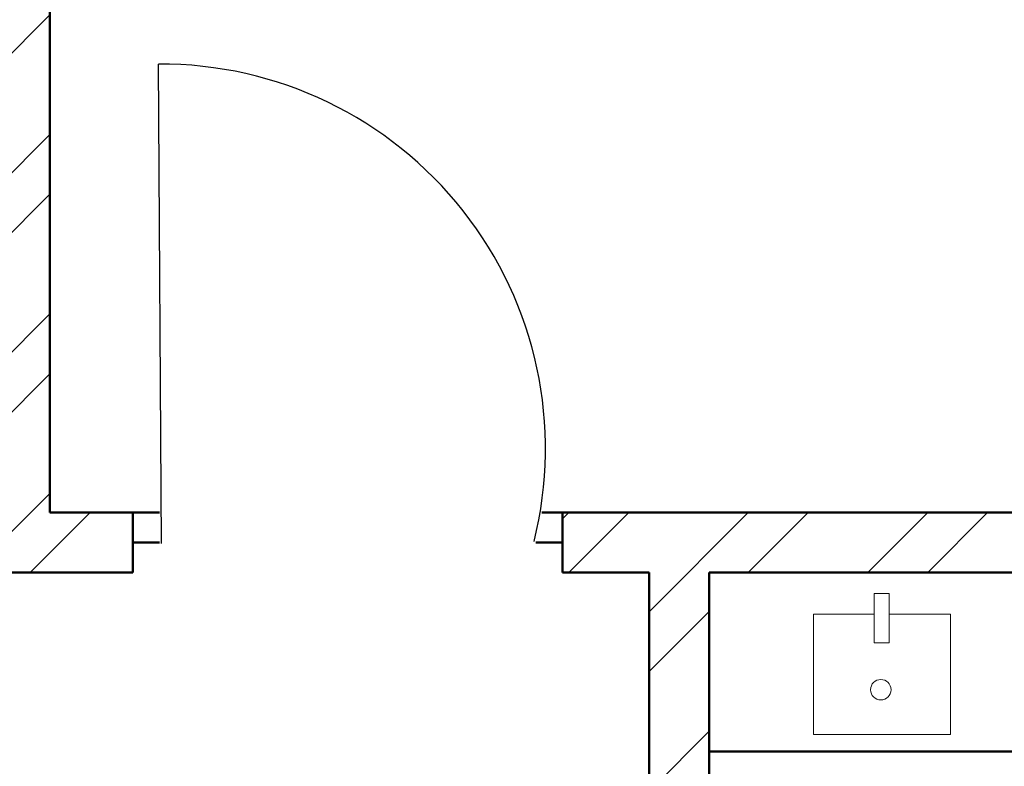
# Model space of a CAD drawing. Units: inches. Extents: x 1901 to 2863, y 888 to 2433.
# Tile 84 of 91: x 2608 to 2682, y 2064 to 2120. Entities that reach past the tile are written whole.
import ezdxf

# ---------------------------------------------------------------- set-up
doc = ezdxf.new("R2010")
doc.units = ezdxf.units.IN
for name, color, linetype, lineweight in [('A-DOOR', 4, 'Continuous', 25), ('A-FLOR-FIXT', 9, 'Continuous', 18), ('A-WALL', 7, 'Continuous', 50), ('A-WALL-PATT', 8, 'Continuous', 13)]:
    doc.layers.add(name, color=color, linetype=linetype, lineweight=lineweight)

# ---------------------------------------------------------------- blocks, each defined once
blk = doc.blocks.new('DOOR-29')
blk.add_line((-0.004, -0.016), (-0.004, 35.984))
blk.add_arc((-0.004, 7.119), 28.865, 345.68885, 90)

msp = doc.modelspace()

# ---------------------------------------------------------------- hatches: boundary and pattern name
at = {"layer": 'A-WALL-PATT'}
h = msp.add_hatch(dxfattribs=at)
h.set_pattern_fill('ANSI32', color=256)
h.paths.add_polyline_path([(2192.501, 2274.134), (2141.264, 2274.134), (2141.264, 2269.634), (2192.501, 2269.634)])
h.paths.add_polyline_path([(2259.926, 2274.134), (2216.501, 2274.134), (2216.501, 2269.634), (2255.426, 2269.634), (2255.426, 2214.634), (2250.809, 2214.634), (2250.809, 2210.134), (2259.926, 2210.134), (2259.926, 2215.134), (2271.756, 2215.134), (2271.756, 2217.384), (2271.756, 2219.634), (2259.926, 2219.634)])
h.paths.add_polyline_path([(2171.426, 2269.634), (2166.926, 2269.634), (2166.926, 2219.634), (2121.238, 2219.634), (2121.238, 2215.134), (2166.926, 2215.134), (2166.926, 2083.134), (2161.807, 2083.134), (2161.807, 2078.634), (2171.426, 2078.634), (2176.996, 2078.634), (2176.996, 2080.884), (2176.996, 2083.134), (2171.426, 2083.134), (2171.426, 2210.134), (2230.912, 2210.134), (2230.912, 2212.384), (2230.912, 2214.634), (2171.426, 2214.634)])
h.paths.add_polyline_path([(2117.264, 2274.134), (2089.426, 2274.134), (2089.426, 2219.634), (2081.136, 2219.634), (2081.136, 2215.134), (2089.426, 2215.134), (2098.004, 2215.134), (2098.004, 2217.384), (2098.004, 2219.634), (2093.926, 2219.634), (2093.926, 2269.634), (2117.264, 2269.634), (2117.264, 2271.884)])
h.paths.add_polyline_path([(2343.426, 2219.634), (2329.295, 2219.634), (2329.295, 2215.134), (2338.926, 2215.134), (2338.926, 2184.739), (2343.426, 2184.739)])
h.paths.add_polyline_path([(2338.926, 2083.134), (2329.295, 2083.134), (2208.966, 2083.134), (2208.966, 2078.634), (2338.926, 2078.634)])
h.paths.add_polyline_path([(2343.426, 2136.739), (2338.926, 2136.739), (2338.926, 1872.634), (2343.426, 1872.634)])
h.paths.add_polyline_path([(2343.426, 1863.634), (2397.68, 1863.634), (2397.68, 1821.634), (2384.138, 1821.634), (2384.138, 1812.634), (2418.33, 1812.634), (2418.33, 1817.134), (2418.33, 1821.634), (2406.68, 1821.634), (2406.68, 1863.634), (2459.499, 1863.634), (2459.499, 1821.634), (2447.138, 1821.634), (2447.138, 1812.634), (2459.499, 1812.634), (2468.499, 1812.634), (2468.499, 1872.634), (2394.426, 1872.634), (2334.426, 1872.634), (2334.426, 1812.634), (2343.426, 1812.634), (2353.251, 1812.634), (2353.251, 1821.634), (2343.426, 1821.634)])
h.paths.add_polyline_path([(2510.014, 1872.634), (2468.499, 1872.634), (2468.499, 1868.134), (2510.014, 1868.134)])
h.paths.add_polyline_path([(2514.009, 1817.134), (2468.499, 1817.134), (2468.499, 1812.634), (2482.114, 1812.634), (2482.114, 1800.606), (2486.614, 1800.606), (2486.614, 1812.634), (2514.009, 1812.634)])
h.paths.add_polyline_path([(2299.247, 1814.884), (2299.247, 1817.134), (2295.926, 1817.134), (2295.926, 1854.169), (2293.676, 1854.169), (2291.426, 1854.169), (2291.426, 1817.134), (2266.109, 1817.134), (2266.109, 1812.634), (2299.247, 1812.634)])
h.paths.add_polyline_path([(2218.109, 1817.134), (2206.46, 1817.134), (2171.426, 1817.134), (2171.426, 1949.134), (2190.1, 1949.134), (2190.1, 1953.634), (2163.468, 1953.634), (2163.468, 1949.134), (2166.926, 1949.134), (2166.926, 1817.134), (2114.297, 1817.134), (2114.297, 1812.634), (2218.109, 1812.634)])
h.paths.add_polyline_path([(2029.426, 1970.922), (2024.926, 1970.922), (2024.926, 1912.717), (2029.426, 1912.717)])
h.paths.add_polyline_path([(2132.297, 1953.634), (2113.926, 1953.634), (2113.926, 1975.888), (2111.676, 1975.888), (2109.426, 1975.888), (2109.426, 1953.634), (2029.426, 1953.634), (2029.426, 1949.134), (2132.297, 1949.134)])
h.paths.add_polyline_path([(2029.426, 1853.606), (2029.31, 1853.606), (2029.31, 1853.606), (2029.426, 1853.606), (2029.426, 1864.717), (2024.926, 1864.717), (2024.926, 1812.634), (2066.297, 1812.634), (2066.297, 1814.884), (2066.297, 1817.134), (2029.426, 1817.134)])
h.paths.add_polyline_path([(2122.926, 2010.088), (2120.676, 2010.088), (2118.426, 2010.088), (2118.426, 2006.134), (2029.426, 2006.134), (2029.426, 2001.634), (2109.426, 2001.634), (2109.426, 1998.041), (2113.926, 1998.041), (2113.926, 2001.634), (2122.926, 2001.634)])
h.paths.add_polyline_path([(2029.426, 2031.376), (2024.926, 2031.376), (2024.926, 1994.922), (2027.176, 1994.922), (2029.426, 1994.922)])
h.paths.add_polyline_path([(2029.426, 2136.739), (2024.926, 2136.739), (2024.926, 2067.376), (2027.176, 2067.376), (2029.426, 2067.376)])
h.paths.add_polyline_path([(2125.618, 2083.134), (2029.426, 2083.134), (2029.426, 2078.634), (2118.426, 2078.634), (2118.426, 2030.715), (2122.926, 2030.715), (2122.926, 2078.634), (2125.618, 2078.634)])
h.paths.add_polyline_path([(2029.426, 2215.134), (2040.468, 2215.134), (2040.468, 2217.384), (2040.468, 2219.634), (2024.926, 2219.634), (2024.926, 2184.739), (2029.426, 2184.739), (2029.426, 2187.778)])
h.paths.add_polyline_path([(2686.426, 2274.134), (2659.284, 2274.134), (2659.284, 2269.634), (2681.926, 2269.634), (2681.926, 2219.634), (2676.816, 2219.634), (2676.816, 2215.134), (2681.926, 2215.134), (2697.011, 2215.134), (2697.011, 2217.384), (2697.011, 2219.634), (2686.426, 2219.634)])
h.paths.add_polyline_path([(2609.926, 2269.634), (2635.284, 2269.634), (2635.284, 2274.134), (2571.431, 2274.134), (2571.431, 2269.634), (2605.426, 2269.634), (2605.426, 2214.634), (2549.098, 2214.634), (2549.098, 2210.134), (2605.426, 2210.134), (2605.426, 2083.134), (2601.014, 2083.134), (2601.014, 2080.884), (2601.014, 2078.634), (2609.926, 2078.634), (2616.162, 2078.634), (2616.162, 2080.884), (2616.162, 2083.134), (2609.926, 2083.134), (2609.926, 2215.134), (2651.465, 2215.134), (2651.465, 2217.384), (2651.465, 2219.634), (2609.926, 2219.634)])
h.paths.add_polyline_path([(2521.426, 2269.634), (2547.431, 2269.634), (2547.431, 2271.884), (2547.431, 2274.134), (2516.926, 2274.134), (2516.926, 2219.634), (2506.41, 2219.634), (2506.41, 2215.134), (2516.926, 2215.134), (2516.926, 2210.134), (2525.402, 2210.134), (2525.402, 2212.384), (2525.402, 2214.634), (2521.426, 2214.634)])
h.paths.add_polyline_path([(2456.011, 2219.634), (2439.426, 2219.634), (2439.426, 2187.888), (2443.926, 2187.888), (2443.926, 2215.134), (2456.011, 2215.134)])
h.paths.add_polyline_path([(2752.926, 2219.634), (2739.485, 2219.634), (2739.485, 2215.134), (2748.426, 2215.134), (2748.426, 2187.888), (2752.926, 2187.888)])
h.paths.add_polyline_path([(2752.926, 2139.888), (2748.426, 2139.888), (2748.426, 2083.134), (2648.416, 2083.134), (2648.416, 2078.634), (2654.926, 2078.634), (2654.926, 2039.437), (2659.426, 2039.437), (2659.426, 2078.634), (2748.426, 2078.634), (2748.426, 2063.429), (2752.926, 2063.429)])
h.paths.add_polyline_path([(2752.926, 2010.634), (2659.426, 2010.634), (2659.426, 2015.652), (2654.926, 2015.652), (2654.926, 2010.634), (2605.426, 2010.634), (2605.426, 1920.967), (2609.926, 1920.967), (2609.926, 2006.134), (2748.426, 2006.134), (2748.426, 1982.466), (2752.926, 1982.466)])
h.paths.add_polyline_path([(2752.926, 2027.429), (2748.426, 2027.429), (2748.426, 2010.634), (2752.926, 2010.634)])
h.paths.add_polyline_path([(2748.426, 1886.134), (2609.926, 1886.134), (2609.926, 1889.719), (2605.426, 1889.719), (2605.426, 1861.262), (2609.926, 1861.262), (2609.926, 1881.634), (2748.426, 1881.634)])
h.paths.add_polyline_path([(2456.855, 2228.831), (2498.401, 2228.831), (2498.401, 2247.488), (2456.855, 2247.488)], flags=9)
h.paths.add_polyline_path([(2038.602, 2237.418), (2080.174, 2237.418), (2080.174, 2256.075), (2038.602, 2256.075)], flags=9)
h.paths.add_polyline_path([(2292.009, 1062.394), (2539.932, 1062.394), (2539.932, 1099.487), (2292.009, 1099.487)], flags=9)
h.paths.add_polyline_path([(2424.91, 1832.253), (2448.513, 1832.253), (2448.513, 1846.678), (2424.91, 1846.678)], flags=25)
h.paths.add_polyline_path([(2359.076, 1832.253), (2382.678, 1832.253), (2382.678, 1846.678), (2359.076, 1846.678)], flags=25)
h.paths.add_polyline_path([(2352.899, 1684.802), (2367.543, 1684.802), (2367.543, 1697.167), (2352.899, 1697.167)], flags=9)
h.paths.add_polyline_path([(2079.288, 1755.826), (2169.024, 1755.826), (2169.024, 1774.372), (2079.288, 1774.372)], flags=9)
h.paths.add_polyline_path([(2404.09, 1373.857), (2404.09, 1463.593), (2385.544, 1463.593), (2385.544, 1373.857)], flags=9)
h.paths.add_polyline_path([(2268.091, 2236.371), (2309.636, 2236.371), (2309.636, 2255.028), (2268.091, 2255.028)], flags=9)
h.paths.add_polyline_path([(2575.96, 1700.951), (2665.696, 1700.951), (2665.696, 1719.498), (2575.96, 1719.498)], flags=9)
h.paths.add_polyline_path([(2302.962, 1878.474), (2329.524, 1878.474), (2329.524, 1888.777), (2302.962, 1888.777)], flags=9)
h.paths.add_polyline_path([(2097.415, 2240.576), (2126.573, 2240.576), (2126.573, 2259.233), (2097.415, 2259.233)], flags=9)
h.paths.add_polyline_path([(2208.725, 2246.124), (2237.882, 2246.124), (2237.882, 2264.781), (2208.725, 2264.781)], flags=9)
h.paths.add_polyline_path([(2038.147, 1925.958), (2076.987, 1925.958), (2076.987, 1944.615), (2038.147, 1944.615)], flags=9)
h.paths.add_polyline_path([(2239.144, 1926.672), (2288.465, 1926.672), (2288.465, 1945.329), (2239.144, 1945.329)], flags=9)
h.paths.add_polyline_path([(2175.429, 2007.33), (2212.356, 2007.33), (2212.356, 2025.987), (2175.429, 2025.987)], flags=9)
h.paths.add_polyline_path([(2225.034, 2091.794), (2263.875, 2091.794), (2263.875, 2110.451), (2225.034, 2110.451)], flags=9)
h.paths.add_polyline_path([(2035.398, 2098.478), (2074.238, 2098.478), (2074.238, 2117.135), (2035.398, 2117.135)], flags=9)
h.paths.add_polyline_path([(2050.102, 2029.209), (2083.26, 2029.209), (2083.26, 2047.866), (2050.102, 2047.866)], flags=9)
h.paths.add_polyline_path([(2069.677, 1956.719), (2098.835, 1956.719), (2098.835, 1975.376), (2069.677, 1975.376)], flags=25)
h.paths.add_polyline_path([(2328.62, 1753.336), (2361.663, 1753.336), (2361.663, 1771.993), (2328.62, 1771.993)], flags=9)
h.paths.add_polyline_path([(2395.162, 2060.888), (2395.162, 2140.654), (2378.676, 2140.654), (2378.676, 2060.888)], flags=9)
h.paths.add_polyline_path([(2463.728, 2059.02), (2492.886, 2059.02), (2492.886, 2077.677), (2463.728, 2077.677)], flags=9)
h.paths.add_polyline_path([(2458.027, 2181.536), (2496.868, 2181.536), (2496.868, 2200.194), (2458.027, 2200.194)], flags=9)
h.paths.add_polyline_path([(2527.577, 2243.074), (2556.735, 2243.074), (2556.735, 2261.731), (2527.577, 2261.731)], flags=9)
h.paths.add_polyline_path([(2694.461, 2232.767), (2736.033, 2232.767), (2736.033, 2251.425), (2694.461, 2251.425)], flags=9)
h.paths.add_polyline_path([(2637.821, 2249.225), (2666.979, 2249.225), (2666.979, 2267.882), (2637.821, 2267.882)], flags=9)
h.paths.add_polyline_path([(2623.687, 2183.541), (2662.528, 2183.541), (2662.528, 2202.199), (2623.687, 2202.199)], flags=9)
h.paths.add_polyline_path([(2691.965, 2021.5), (2725.124, 2021.5), (2725.124, 2040.157), (2691.965, 2040.157)], flags=9)
h.paths.add_polyline_path([(2621.043, 1975.912), (2662.335, 1975.912), (2662.335, 1994.569), (2621.043, 1994.569)], flags=25)
h.paths.add_polyline_path([(2479.032, 1927.62), (2519.844, 1927.62), (2519.844, 1946.277), (2479.032, 1946.277)], flags=9)
h.paths.add_polyline_path([(2670.941, 1849.076), (2716.005, 1849.076), (2716.005, 1867.734), (2670.941, 1867.734)], flags=9)
h.paths.add_polyline_path([(2523.613, 1782.956), (2550.175, 1782.956), (2550.175, 1793.26), (2523.613, 1793.26)], flags=9)
h.paths.add_polyline_path([(2450.841, 1207.331), (2492.386, 1207.331), (2492.386, 1225.989), (2450.841, 1225.989)], flags=9)
h.paths.add_polyline_path([(2527.751, 1203.841), (2556.908, 1203.841), (2556.908, 1222.499), (2527.751, 1222.499)], flags=9)
h.paths.add_polyline_path([(2639.111, 1207.2), (2668.268, 1207.2), (2668.268, 1225.857), (2639.111, 1225.857)], flags=9)
h.paths.add_polyline_path([(2692.594, 1218.965), (2734.167, 1218.965), (2734.167, 1237.623), (2692.594, 1237.623)], flags=9)
h.paths.add_polyline_path([(2669.266, 1366.329), (2708.106, 1366.329), (2708.106, 1384.987), (2669.266, 1384.987)], flags=9)
h.paths.add_polyline_path([(2463.313, 1358.031), (2502.153, 1358.031), (2502.153, 1376.688), (2463.313, 1376.688)], flags=9)
h.paths.add_polyline_path([(2494.725, 1449.963), (2531.652, 1449.963), (2531.652, 1468.62), (2494.725, 1468.62)], flags=9)
h.paths.add_polyline_path([(2675.565, 1422.157), (2708.724, 1422.157), (2708.724, 1440.815), (2675.565, 1440.815)], flags=9)
h.paths.add_polyline_path([(2685.634, 1493.891), (2714.792, 1493.891), (2714.792, 1512.548), (2685.634, 1512.548)], flags=9)
h.paths.add_polyline_path([(2686.805, 1529.913), (2725.645, 1529.913), (2725.645, 1548.57), (2686.805, 1548.57)], flags=9)
h.paths.add_polyline_path([(2503.651, 1537.991), (2552.972, 1537.991), (2552.972, 1556.648), (2503.651, 1556.648)], flags=9)
h.paths.add_polyline_path([(2291.713, 1643.504), (2318.275, 1643.504), (2318.275, 1653.807), (2291.713, 1653.807)], flags=9)
h.paths.add_polyline_path([(2450.626, 1610.52), (2477.189, 1610.52), (2477.189, 1620.824), (2450.626, 1620.824)], flags=9)
h.paths.add_polyline_path([(2359.985, 1551.814), (2422.253, 1551.814), (2422.253, 1562.117), (2359.985, 1562.117)], flags=9)
h.paths.add_polyline_path([(2280.106, 1249.006), (2321.651, 1249.006), (2321.651, 1267.663), (2280.106, 1267.663)], flags=9)
h.paths.add_polyline_path([(2164.057, 1274.232), (2193.215, 1274.232), (2193.215, 1292.889), (2164.057, 1292.889)], flags=9)
h.paths.add_polyline_path([(2118.21, 1277.694), (2151.252, 1277.694), (2151.252, 1296.351), (2118.21, 1296.351)], flags=9)
h.paths.add_polyline_path([(2031.946, 1268.529), (2073.519, 1268.529), (2073.519, 1287.187), (2031.946, 1287.187)], flags=9)
h.paths.add_polyline_path([(2050.199, 1409.079), (2089.04, 1409.079), (2089.04, 1427.736), (2050.199, 1427.736)], flags=9)
h.paths.add_polyline_path([(2243.743, 1421.032), (2282.584, 1421.032), (2282.584, 1439.689), (2243.743, 1439.689)], flags=9)
h.paths.add_polyline_path([(2190.746, 1509.769), (2231.558, 1509.769), (2231.558, 1528.426), (2190.746, 1528.426)], flags=9)
h.paths.add_polyline_path([(2058.392, 1475.415), (2091.55, 1475.415), (2091.55, 1494.073), (2058.392, 1494.073)], flags=9)
h.paths.add_polyline_path([(2062.447, 1553.09), (2091.605, 1553.09), (2091.605, 1571.747), (2062.447, 1571.747)], flags=9)
h.paths.add_polyline_path([(2219.524, 1590.365), (2266.147, 1590.365), (2266.147, 1609.022), (2219.524, 1609.022)], flags=9)
h.paths.add_polyline_path([(2041.072, 1584.188), (2079.912, 1584.188), (2079.912, 1602.845), (2041.072, 1602.845)], flags=9)

# ---------------------------------------------------------------- linework, layer by layer
at = {"layer": 'A-FLOR-FIXT'}
msp.add_lwpolyline([(2671.81, 2077.052), (2672.939, 2077.052), (2672.939, 2073.356), (2671.81, 2073.356)], close=True, dxfattribs=at)
msp.add_lwpolyline([(2672.939, 2075.522), (2677.53, 2075.522), (2677.53, 2066.473), (2667.256, 2066.473), (2667.256, 2075.522), (2671.81, 2075.522)], dxfattribs=at)
msp.add_circle((2672.302, 2069.841), 0.768, dxfattribs=at)
at = {"layer": 'A-WALL'}
for p, q in [((2609.926, 2215.134), (2609.926, 2083.134)), ((2609.926, 2083.134), (2618.162, 2083.134)), ((2609.926, 2083.134), (2618.162, 2083.134)), ((2616.162, 2083.134), (2616.162, 2078.634)), ((2646.874, 2083.134), (2651.465, 2083.134)), ((2646.874, 2083.134), (2748.426, 2083.134)), ((2648.416, 2083.134), (2648.416, 2078.634)), ((2616.162, 2078.634), (2616.162, 2080.884)), ((2616.162, 2080.884), (2618.162, 2080.884)), ((2648.416, 2080.884), (2646.416, 2080.884)), ((2648.416, 2078.634), (2648.416, 2080.884)), ((2601.014, 2078.634), (2609.926, 2078.634)), ((2609.926, 2078.634), (2616.162, 2078.634)), ((2648.416, 2078.634), (2654.926, 2078.634)), ((2654.926, 2078.634), (2654.926, 2039.437)), ((2659.426, 2078.634), (2748.426, 2078.634)), ((2659.426, 2037.744), (2659.426, 2078.634)), ((2659.426, 2067.976), (2659.426, 2067.976)), ((2659.426, 2065.199), (2659.426, 2065.199)), ((2659.426, 2065.199), (2734.984, 2065.199))]:
    msp.add_line(p, q, dxfattribs=at)

# ---------------------------------------------------------------- block references
at = {"layer": 'A-DOOR', "rotation": 0.349108383739448}
msp.add_blockref('DOOR-29', (2618.319, 2080.822), dxfattribs=at)

doc.saveas('drawing.dxf')
